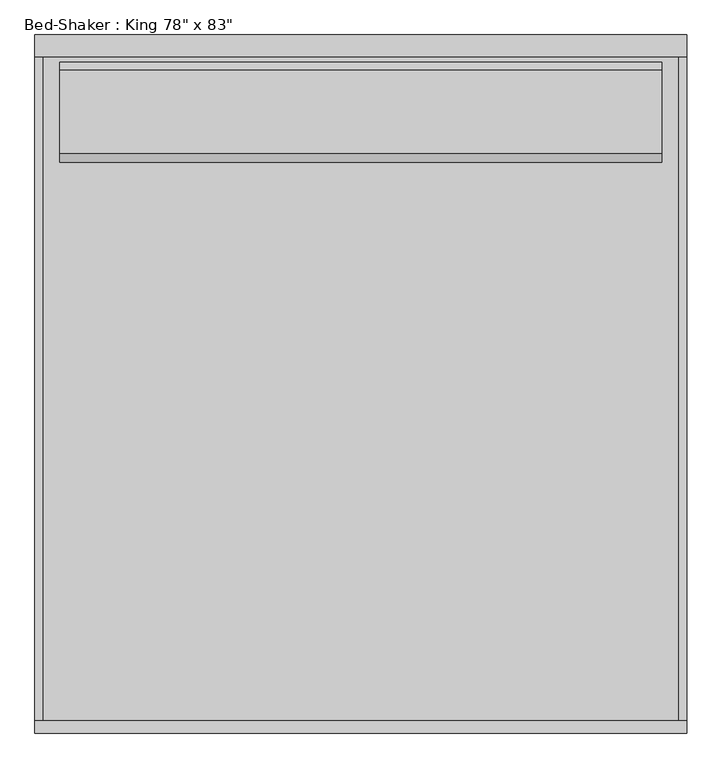
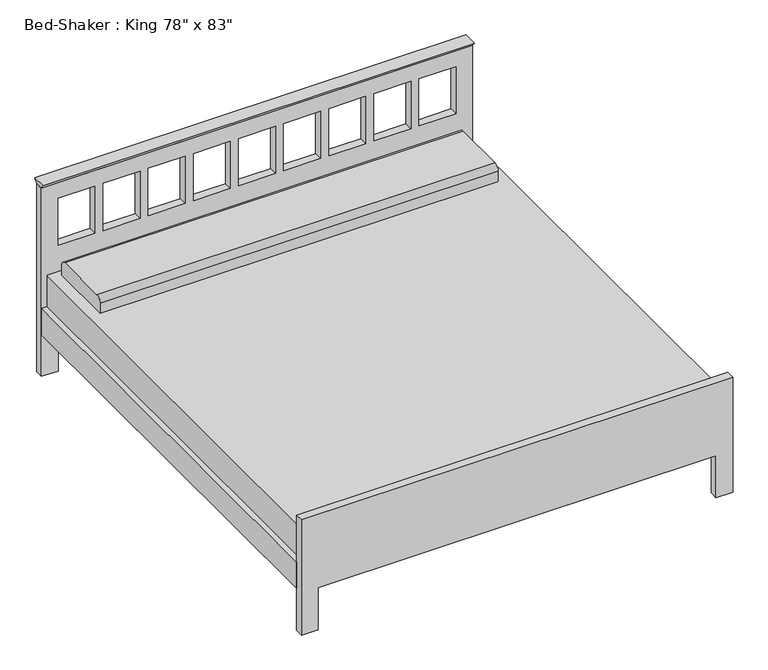
"""IFC4 building model written with IfcOpenShell, lengths in millimetres: furniture geometry."""

from ifc_helpers import new_model, si_unit, point, frame, frame_2d, origin, place, context, project, spatial, polyline, circle_curve, trimmed, segment, composite_curve, outline, extrude, source, transform, mapped, element, save


def furniture_29cd36cd(model_context):
    return source(origin(), model_context, "Body", "SweptSolid", [
        extrude(outline(polyline([(-38.1, 914.4), (-51.9545455, 933.45), (13.8545455, 933.45), (0.0, 914.4), (-38.1, 914.4)])), frame((-1009.4365546, 0.0, 0.0), z_axis=(1.0, 0.0, 0.0), x_axis=(0.0, 1.0, 0.0)), (0.0, 0.0, 1.0), 1981.2533613),
        extrude(outline(composite_curve([segment(polyline([(-373.2486637, 482.6), (-373.2486637, 533.4)]), True, "CONTINUOUS"), segment(trimmed(circle_curve(frame_2d((-347.8486637, 533.4)), 25.4), [point((-373.2486637, 533.4))], [point((-347.8486637, 558.8))], False, "CARTESIAN"), True, "CONTINUOUS"), segment(polyline([(-347.8486637, 558.8), (-93.8486637, 558.8)]), True, "CONTINUOUS"), segment(trimmed(circle_curve(frame_2d((-93.8486637, 533.4)), 25.4), [point((-93.8486637, 558.8))], [point((-68.4486637, 533.4))], False, "CARTESIAN"), True, "CONTINUOUS"), segment(polyline([(-68.4486637, 533.4), (-68.4486637, 482.6), (-373.2486637, 482.6)]), True, "CONTINUOUS")], self_intersect=False)), frame((-933.45, 0.0, 0.0), z_axis=(1.0, 0.0, 0.0), x_axis=(0.0, 1.0, 0.0)), (0.0, 0.0, 1.0), 1828.8),
        extrude(outline(polyline([(946.15, -38.1), (946.15, -2070.1), (-984.25, -2070.1), (-984.25, -38.1), (946.15, -38.1)])), frame((0.0, 0.0, 228.6), z_axis=(0.0, 0.0, 1.0), x_axis=(1.0, 0.0, 0.0)), (0.0, 0.0, 1.0), 254.0),
        extrude(outline(polyline([(946.15, -2070.1), (946.15, -38.1), (971.55, -38.1), (971.55, -2070.1), (946.15, -2070.1)])), frame((0.0, 0.0, 203.0994861), z_axis=(0.0, 0.0, 1.0), x_axis=(1.0, 0.0, 0.0)), (0.0, 0.0, 1.0), 127.0),
        extrude(outline(polyline([(-1009.65, -2070.1), (-1009.65, -38.1), (-984.25, -38.1), (-984.25, -2070.1), (-1009.65, -2070.1)])), frame((0.0, 0.0, 203.5755296), z_axis=(0.0, 0.0, 1.0), x_axis=(1.0, 0.0, 0.0)), (0.0, 0.0, 1.0), 127.0),
        extrude(outline(polyline([(0.0, -933.45), (203.2, -933.45), (203.2, 895.35), (0.0, 895.35), (0.0, 971.55), (558.8, 971.55), (558.8, -1009.65), (0.0, -1009.65), (0.0, -933.45)])), frame((0.0, -2108.2, 0.0), z_axis=(0.0, 1.0, 0.0), x_axis=(0.0, 0.0, 1.0)), (0.0, 0.0, 1.0), 38.1),
        extrude(outline(polyline([(914.4, 971.8168067), (914.4, -1009.4365546), (0.0, -1009.4365546), (0.0, -933.45), (203.2, -933.45), (203.2, 895.35), (0.0, 895.35), (0.0, 971.8168067), (914.4, 971.8168067)]), holes=[polyline([(838.2, -764.1166667), (609.6, -764.1166667), (609.6, -933.45), (838.2, -933.45), (838.2, -764.1166667)]), polyline([(838.2, -556.6833333), (609.6, -556.6833333), (609.6, -726.0166667), (838.2, -726.0166667), (838.2, -556.6833333)]), polyline([(838.2, -349.25), (609.6, -349.25), (609.6, -518.5833333), (838.2, -518.5833333), (838.2, -349.25)]), polyline([(838.2, -141.8166667), (609.6, -141.8166667), (609.6, -311.15), (838.2, -311.15), (838.2, -141.8166667)]), polyline([(838.2, 273.05), (609.6, 273.05), (609.6, 103.7166667), (838.2, 103.7166667), (838.2, 273.05)]), polyline([(838.2, 480.4833333), (609.6, 480.4833333), (609.6, 311.15), (838.2, 311.15), (838.2, 480.4833333)]), polyline([(838.2, 687.9166667), (609.6, 687.9166667), (609.6, 518.5833333), (838.2, 518.5833333), (838.2, 687.9166667)]), polyline([(838.2, 895.35), (609.6, 895.35), (609.6, 726.0166667), (838.2, 726.0166667), (838.2, 895.35)]), polyline([(838.2, 65.6166667), (609.6, 65.6166667), (609.6, -103.7166667), (838.2, -103.7166667), (838.2, 65.6166667)])]), frame((0.0, -38.1, 0.0), z_axis=(0.0, 1.0, 0.0), x_axis=(0.0, 0.0, 1.0)), (0.0, 0.0, 1.0), 38.1),
    ])


if __name__ == "__main__":
    model = new_model("IFC4")
    model_context = context("Model", 3, world=origin())
    ifc_project = project(units=[si_unit("LENGTHUNIT", "METRE", prefix="MILLI")], contexts=[model_context])
    site = spatial("IfcSite", under=ifc_project)
    building = spatial("IfcBuilding", under=site)
    placement = place(None, origin())
    furniture_shape = furniture_29cd36cd(model_context)
    element("IfcFurniture", 1, ObjectType="Bed-Shaker : King 78\" x 83\"", at=placement, inside=building, context=model_context, shape_type="MappedRepresentation", body=[
        mapped(furniture_shape, transform((0.0, 0.0, 0.0), x_axis=(1.0, 0.0, 0.0), y_axis=(0.0, 1.0, 0.0), z_axis=(0.0, 0.0, 1.0))),
    ])
    save(model, "model.ifc")

# Revit data of these elements
# Type "Bed-Shaker : King 78\" x 83\""
#   Assembly Code = "E2020200"
#   Length = 6' - 11"
#   Width = 6' - 6"
#   Frame Material = Birch
#   Mattress Material = Linen, White
#   Default Elevation = 0
# Element 1 (IfcFurniture, "Bed-Shaker : King 78\" x 83\"")
#   Materials on its faces: "Birch", "Linen, White"
# Materials
#   "Birch": class "Wood", colour RGB 224 178 126, transparency 0, Description = "Betula Alleghaniensis", Cost = 0
#   "Linen, White": class "Textile", colour RGB 247 247 239, transparency 0, Description = "Linen, white", Cost = 0
